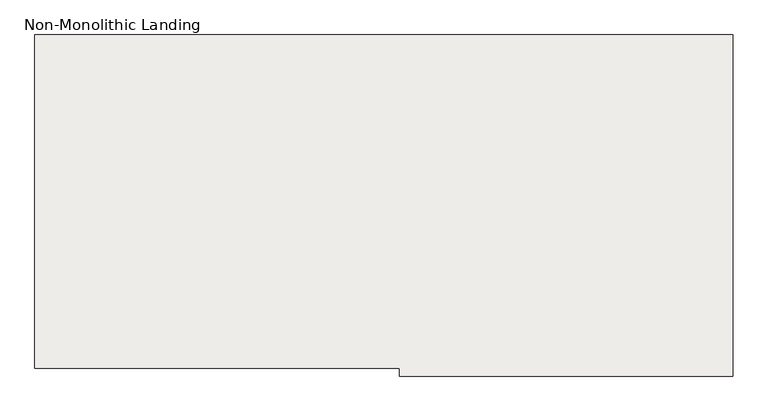
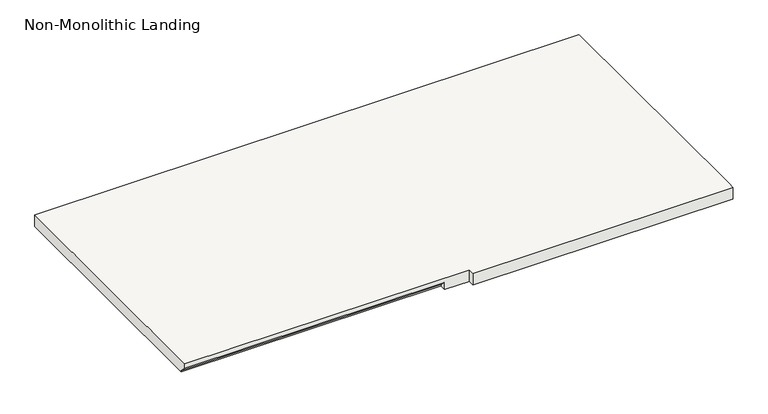
"""IFC4 building model written with IfcOpenShell, lengths in millimetres: slab geometry, Non-Monolithic Landing."""

from ifc_helpers import new_model, si_unit, origin, place, context, project, spatial, faceted_brep, source, transform, mapped, element, save


def non_monolithic_landing_dd6d84fa(model_context):
    return source(origin(), model_context, "Body", "Brep", [
        faceted_brep([(-6252.9338869, 4855.3468856, 1906.0026316), (-6252.9338869, 4880.7468856, 1880.6026316), (-5186.1338869, 4880.7468856, 1880.6026316), (-5186.1338869, 4855.3468856, 1906.0026316), (-5084.5338869, 4855.3468856, 1925.0526316), (-5084.5338869, 4829.9468856, 1925.0526316), (-4017.7338869, 4829.9468856, 1925.0526316), (-4017.7338869, 4855.3468856, 1925.0526316), (-4017.7338869, 5922.1468856, 1925.0526316), (-6252.9338869, 5922.1468856, 1925.0526316), (-6252.9338869, 4855.3468856, 1925.0526316), (-5186.1338869, 4880.7468856, 1874.2526316), (-6252.9338869, 4880.7468856, 1874.2526316), (-6252.9338869, 5922.1468856, 1874.2526316), (-4017.7338869, 5922.1468856, 1874.2526316), (-4017.7338869, 4855.3468856, 1874.2526316), (-4017.7338869, 4829.9468856, 1874.2526316), (-5084.5338869, 4829.9468856, 1874.2526316), (-5084.5338869, 4855.3468856, 1874.2526316), (-5186.1338869, 4855.3468856, 1874.2526316)], [[[0, 1, 2, 3]], [[4, 5, 6, 7, 8, 9, 10]], [[11, 12, 13, 14, 15, 16, 17, 18, 19]], [[12, 11, 2, 1]], [[11, 19, 3, 2]], [[4, 10, 0, 3, 19, 18]], [[5, 4, 18, 17]], [[6, 5, 17, 16]], [[7, 6, 16, 15]], [[8, 7, 15, 14]], [[9, 8, 14, 13]], [[10, 9, 13, 12, 1, 0]]]),
    ])


if __name__ == "__main__":
    model = new_model("IFC4")
    model_context = context("Model", 3, world=origin())
    ifc_project = project(units=[si_unit("LENGTHUNIT", "METRE", prefix="MILLI")], contexts=[model_context])
    site = spatial("IfcSite", under=ifc_project)
    building = spatial("IfcBuilding", under=site)
    placement = place(None, origin())
    non_monolithic_landing_shape = non_monolithic_landing_dd6d84fa(model_context)
    element("IfcSlab", 1, ObjectType="Non-Monolithic Landing", at=placement, inside=building, context=model_context, shape_type="MappedRepresentation", body=[
        mapped(non_monolithic_landing_shape, transform((0.0, 0.0, 0.0), x_axis=(1.0, 0.0, 0.0), y_axis=(0.0, 1.0, 0.0), z_axis=(0.0, 0.0, 1.0))),
    ])
    save(model, "model.ifc")
